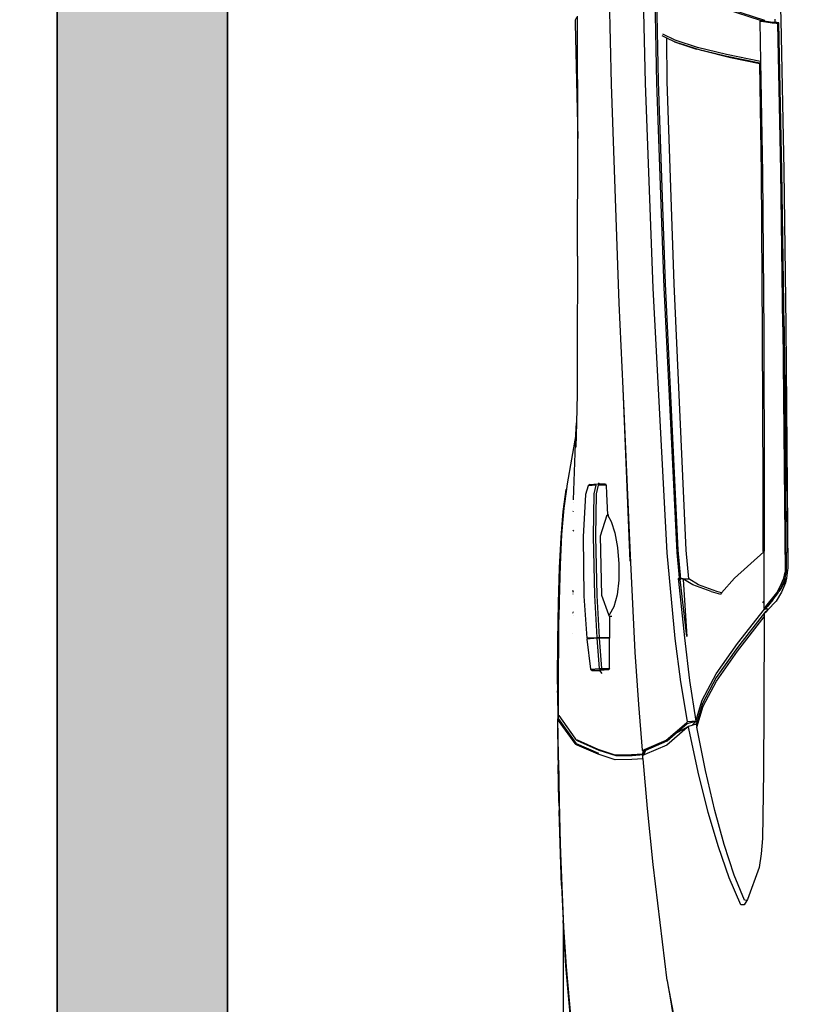
# Model space of a CAD drawing. Units: inches. Extents: x -4737294 to -4736756, y 1716389 to 1717040.
# Tile 7 of 25: x -4737217 to -4737176, y 1716491 to 1716543. Entities that reach past the tile are written whole.
import ezdxf

# ---------------------------------------------------------------- set-up
doc = ezdxf.new("R2010")
doc.units = ezdxf.units.IN
doc.header["$MEASUREMENT"] = 0
for name, color, linetype, lineweight in [('A-ANNO-DIMS', 2, 'Continuous', 18), ('A-EQPM-VEHI', 250, 'Continuous', 13), ('A-WALL-PATT', 244, 'Continuous', 13), ('walls', 252, 'Continuous', 35)]:
    doc.layers.add(name, color=color, linetype=linetype, lineweight=lineweight)
doc.layers.add('Edges', color=250, linetype='Continuous')
doc.styles.get("Standard").update_dxf_attribs({"font": 'arial.ttf'})
doc.dimstyles.get("Standard").update_dxf_attribs({"dimtxt": 8, "dimasz": 0.18, "dimexe": 0.18, "dimexo": 0.0625, "dimgap": 0.09, "dimtad": 0, "dimtih": 1, "dimtoh": 1, "dimzin": 0, "dimdsep": 46, "dimlunit": 3, "dimtxsty": 'Standard', "dimcen": 0.09, "dimadec": 0, "dimazin": 0, "dimtfac": 1, "dimtofl": 0, "dimtmove": 0, "dimatfit": 3, "dimfxl": 1, "dimtolj": 1, "dimtzin": 0, "dimarcsym": 0})

# ---------------------------------------------------------------- blocks, each defined once
blk = doc.blocks.new('Nissan Qashqai pl')
at = {"layer": 'Edges'}
for p, q in [((10.2357, 11.3043), (10.53, 11.3068)), ((10.4182, 11.3058), (10.53, 11.3068)), ((10.53, 11.3068), (10.5301, 11.3068)), ((10.5301, 11.3068), (10.5323, 11.3065)), ((10.5323, 11.3065), (10.5419, 11.3051)), ((9.696, 11.2932), (9.8644, 11.2982)), ((9.8644, 11.2982), (10.0472, 11.3018)), ((9.8681, 11.2959), (9.8678, 11.2935)), ((10.0476, 11.2996), (9.8681, 11.2959)), ((9.8681, 11.2959), (9.869, 11.2946)), ((9.869, 11.2946), (9.8689, 11.2927)), ((10.0477, 11.2982), (9.869, 11.2946)), ((10.0472, 11.3018), (10.2357, 11.3043)), ((10.2367, 11.3022), (10.0476, 11.2996)), ((10.2369, 11.3008), (10.0477, 11.2982)), ((10.2367, 11.3022), (10.5351, 11.305)), ((10.2369, 11.3008), (10.5348, 11.3036)), ((10.4153, 11.3058), (10.2954, 11.3046)), ((10.4153, 11.3058), (10.4174, 11.3058)), ((10.4174, 11.3058), (10.4181, 11.3058)), ((10.4181, 11.3058), (10.4182, 11.3058)), ((10.5422, 11.3021), (10.5348, 11.3036)), ((10.5424, 11.3035), (10.5351, 11.305)), ((10.5366, 11.3048), (10.536, 11.305)), ((10.5379, 11.3052), (10.5381, 11.305)), ((10.5419, 11.3051), (10.5463, 11.3031)), ((10.5419, 11.3051), (10.5479, 11.3042)), ((10.5522, 11.2977), (10.5422, 11.3021)), ((10.5472, 11.3014), (10.5424, 11.3035)), ((10.5463, 11.3031), (10.5551, 11.2984)), ((10.5546, 11.2982), (10.5472, 11.3014)), ((10.5479, 11.3042), (10.5589, 11.2991)), ((10.5598, 11.2935), (10.5522, 11.2977)), ((10.5583, 11.296), (10.5546, 11.2982)), ((10.5551, 11.2984), (10.5583, 11.296)), ((10.5612, 11.2944), (10.5583, 11.296)), ((10.5589, 11.2991), (10.57, 11.2925)), ((10.5683, 11.2885), (10.5612, 11.2944)), ((9.8637, 11.291), (9.8643, 11.291)), ((9.8643, 11.291), (9.8677, 11.291)), ((9.8675, 11.2887), (9.8655, 11.2754)), ((9.8686, 11.2879), (9.8665, 11.2747)), ((9.8677, 11.291), (9.8675, 11.2887)), ((9.8678, 11.2935), (9.8677, 11.291)), ((9.8689, 11.2927), (9.8686, 11.2879)), ((10.5764, 11.28), (10.5598, 11.2935)), ((10.5683, 11.2885), (10.573, 11.285)), ((10.575, 11.2829), (10.5683, 11.2885)), ((10.57, 11.2925), (10.5811, 11.2822)), ((10.573, 11.285), (10.5769, 11.2818)), ((10.5776, 11.2808), (10.575, 11.2829)), ((10.5796, 11.2824), (10.5796, 11.2787)), ((10.5811, 11.2822), (10.5821, 11.2808)), ((10.5811, 11.2822), (10.5834, 11.28)), ((9.8652, 11.2788), (9.8516, 11.2363)), ((9.8652, 11.2738), (9.8516, 11.2313)), ((9.8652, 11.2738), (9.8652, 11.2788)), ((9.8655, 11.2754), (9.8652, 11.2738)), ((9.8652, 11.2735), (9.8665, 11.2747)), ((9.8652, 11.2738), (9.8652, 11.2738)), ((9.8652, 11.2738), (9.8652, 11.2735)), ((9.8652, 11.2735), (9.8664, 11.2728)), ((9.8665, 11.2747), (9.8664, 11.2728)), ((9.8664, 11.2728), (9.9149, 11.2736)), ((9.9149, 11.2736), (9.9066, 11.2322)), ((9.9169, 11.2728), (9.9086, 11.2313)), ((9.9177, 11.2728), (9.9106, 11.2373)), ((9.9149, 11.2736), (10.0505, 11.276)), ((9.9177, 11.2728), (9.9169, 11.2728)), ((10.0501, 11.2747), (9.9177, 11.2728)), ((10.2453, 11.2762), (10.0501, 11.2747)), ((10.0505, 11.276), (10.2453, 11.2777)), ((10.2453, 11.2777), (10.4289, 11.2783)), ((10.4292, 11.2767), (10.2453, 11.2762)), ((10.4289, 11.2783), (10.5092, 11.2783)), ((10.5099, 11.2768), (10.4292, 11.2767)), ((10.5099, 11.2768), (10.5092, 11.2783)), ((10.5092, 11.2783), (10.5094, 11.2783)), ((10.5094, 11.2783), (10.51, 11.2776)), ((10.5783, 11.2783), (10.5094, 11.2783)), ((10.51, 11.2776), (10.5099, 11.2768)), ((10.51, 11.2776), (10.5419, 11.2423)), ((10.5705, 11.2771), (10.5709, 11.2767)), ((10.5709, 11.2767), (10.5719, 11.2759)), ((10.5783, 11.2783), (10.5764, 11.28)), ((10.5796, 11.2787), (10.5776, 11.2808)), ((10.5776, 11.2808), (10.5783, 11.2783)), ((10.5796, 11.2787), (10.5783, 11.2783)), ((10.6215, 11.2456), (10.5796, 11.2787)), ((10.5821, 11.2808), (10.5834, 11.2793)), ((10.5825, 11.2806), (10.5834, 11.2793)), ((10.5834, 11.28), (10.5851, 11.2783)), ((10.5834, 11.2793), (10.5835, 11.2793)), ((10.5835, 11.2793), (10.584, 11.2787)), ((10.584, 11.2789), (10.584, 11.2793)), ((10.584, 11.2787), (10.584, 11.2789)), ((10.584, 11.2787), (10.6261, 11.2458)), ((10.584, 11.2787), (10.5851, 11.2783)), ((10.5843, 11.2787), (10.584, 11.2787)), ((10.5847, 11.2787), (10.5843, 11.2787)), ((10.5851, 11.2783), (10.5892, 11.2783)), ((10.6306, 11.2459), (10.5892, 11.2783)), ((10.5892, 11.2783), (10.6988, 11.2779)), ((10.6988, 11.2779), (10.7769, 11.2774)), ((10.7769, 11.2774), (10.858, 11.2759)), ((10.858, 11.2759), (10.8766, 11.2745)), ((10.8766, 11.2745), (10.8932, 11.2722)), ((10.8932, 11.2722), (10.932, 11.258)), ((10.932, 11.258), (10.9335, 11.257)), ((10.933, 11.2541), (10.9026, 11.2417)), ((10.9384, 11.2497), (10.9059, 11.2355)), ((10.9335, 11.257), (10.933, 11.2541)), ((10.9335, 11.257), (10.9386, 11.2537)), ((10.9386, 11.2537), (10.9384, 11.2497)), ((9.9106, 11.2373), (9.9018, 11.2021)), ((10.5419, 11.2423), (10.56, 11.2265)), ((10.6583, 11.2197), (10.6215, 11.2456)), ((10.6261, 11.2458), (10.6627, 11.22)), ((10.6671, 11.2203), (10.6306, 11.2459)), ((10.9026, 11.2417), (10.8653, 11.2297)), ((10.9059, 11.2355), (10.8682, 11.2226)), ((9.9066, 11.2322), (9.8978, 11.197)), ((9.9086, 11.2313), (9.8998, 11.196)), ((10.56, 11.2265), (10.5584, 11.2206)), ((10.5584, 11.2136), (10.5617, 11.2251)), ((10.56, 11.2265), (10.5617, 11.2251)), ((10.8653, 11.2297), (10.8239, 11.2181)), ((10.8682, 11.2226), (10.8264, 11.21)), ((10.5584, 11.2206), (10.5502, 11.1986)), ((10.5584, 11.2136), (10.5502, 11.1916)), ((10.69, 11.2028), (10.6583, 11.2197)), ((10.6627, 11.22), (10.6943, 11.2032)), ((10.6976, 11.2041), (10.6671, 11.2203)), ((10.8239, 11.2181), (10.7754, 11.2071)), ((9.9018, 11.2021), (9.8931, 11.1752)), ((10.5502, 11.1986), (10.543, 11.1865)), ((10.7155, 11.1952), (10.69, 11.2028)), ((10.6943, 11.2032), (10.7155, 11.1969)), ((10.7228, 11.1965), (10.6976, 11.2041)), ((10.7754, 11.2071), (10.7228, 11.1965)), ((10.8264, 11.21), (10.7776, 11.1982)), ((9.8978, 11.197), (9.8891, 11.1701)), ((9.8911, 11.1693), (9.8998, 11.196)), ((10.543, 11.1865), (10.5079, 11.1835)), ((10.5502, 11.1916), (10.543, 11.1795)), ((10.543, 11.1795), (10.543, 11.1865)), ((10.6144, 11.1813), (10.6664, 11.1875)), ((10.6664, 11.1875), (10.7155, 11.1952)), ((10.7155, 11.1957), (10.7155, 11.1969)), ((10.7155, 11.1969), (10.7192, 11.1957)), ((10.7209, 11.1902), (10.7155, 11.1957)), ((10.7155, 11.1952), (10.7155, 11.1957)), ((10.7186, 11.1848), (10.7155, 11.1952)), ((10.7155, 11.1952), (10.7165, 11.1851)), ((10.7192, 11.1957), (10.7228, 11.1965)), ((10.7192, 11.1957), (10.7209, 11.1902)), ((10.7209, 11.1902), (10.7221, 11.1861)), ((10.7247, 11.1867), (10.7222, 11.186)), ((10.7776, 11.1982), (10.7247, 11.1867)), ((9.8931, 11.1751), (9.8911, 11.1693)), ((9.8931, 11.1751), (9.8931, 11.1752)), ((10.5079, 11.1835), (10.1849, 11.1687)), ((10.543, 11.1771), (10.5079, 11.1739)), ((10.5109, 11.1721), (10.5417, 11.1748)), ((10.543, 11.1771), (10.5417, 11.1748)), ((10.5417, 11.1748), (10.5427, 11.1739)), ((10.5436, 11.1754), (10.5427, 11.1739)), ((10.5439, 11.1796), (10.543, 11.1795)), ((10.543, 11.1795), (10.543, 11.1771)), ((10.544, 11.1763), (10.543, 11.1771)), ((10.544, 11.1763), (10.5436, 11.1754)), ((10.5439, 11.1796), (10.613, 11.1841)), ((10.547, 11.1767), (10.544, 11.1763)), ((10.5458, 11.1742), (10.6144, 11.1813)), ((10.613, 11.1841), (10.547, 11.1767)), ((10.6678, 11.177), (10.6152, 11.1702)), ((10.7137, 11.1846), (10.6678, 11.177)), ((10.7165, 11.1851), (10.7137, 11.1846)), ((10.7177, 11.1838), (10.7165, 11.1851)), ((10.7387, 11.1593), (10.7177, 11.1838)), ((10.7312, 11.1701), (10.7186, 11.1848)), ((10.7221, 11.1861), (10.7222, 11.1859)), ((10.7222, 11.186), (10.7221, 11.1861)), ((10.7222, 11.186), (10.7222, 11.1859)), ((10.7222, 11.1859), (10.7232, 11.1848)), ((10.7222, 11.1859), (10.7224, 11.1855)), ((10.7224, 11.1855), (10.7312, 11.1701)), ((10.7232, 11.1848), (10.7228, 11.1859)), ((10.7232, 11.1848), (10.7449, 11.1598)), ((10.7257, 11.1853), (10.7256, 11.1854)), ((11.0357, 11.1613), (11.1598, 11.1847)), ((11.0492, 11.1635), (11.1336, 11.1772)), ((9.8891, 11.1701), (9.8818, 11.1551)), ((9.8911, 11.1691), (9.8867, 11.16)), ((9.8911, 11.1693), (9.8911, 11.1691)), ((10.1849, 11.1687), (9.9393, 11.1602)), ((10.5079, 11.1739), (10.1849, 11.1585)), ((10.1894, 11.1563), (10.5109, 11.1721)), ((10.6152, 11.1702), (10.5113, 11.1603)), ((10.5427, 11.1739), (10.5458, 11.1742)), ((10.7397, 11.1602), (10.7312, 11.1701)), ((11.0357, 11.1613), (11.0491, 11.1635)), ((11.0492, 11.1635), (11.0491, 11.1635)), ((9.8867, 11.16), (9.8838, 11.1541)), ((9.9393, 11.1602), (9.8867, 11.16)), ((10.1849, 11.1585), (9.9393, 11.1497)), ((9.9411, 11.1475), (10.1894, 11.1563)), ((10.5113, 11.1603), (10.19, 11.1433)), ((10.7501, 11.1327), (10.7387, 11.1593)), ((10.7507, 11.1344), (10.7397, 11.1602)), ((10.7449, 11.1598), (10.7563, 11.1333)), ((11.0304, 11.1603), (10.8896, 11.1434)), ((11.0304, 11.1603), (11.0357, 11.1613)), ((9.8101, 11.1449), (9.9411, 11.1475)), ((9.9393, 11.1497), (9.8119, 11.1472)), ((10.19, 11.1433), (9.9414, 11.1341)), ((10.8896, 11.1434), (10.8218, 11.1365)), ((9.9414, 11.1341), (9.8143, 11.1312)), ((10.6955, 11.1257), (10.7509, 11.1302)), ((10.7507, 11.1309), (10.7501, 11.1327)), ((10.7511, 11.1335), (10.7507, 11.1344)), ((10.7507, 11.1344), (10.7524, 11.1335)), ((10.751, 11.131), (10.7507, 11.1309)), ((10.7509, 11.1302), (10.7507, 11.1309)), ((10.7522, 11.1311), (10.7509, 11.1302)), ((10.7516, 11.131), (10.7509, 11.1302)), ((10.7519, 11.1314), (10.7511, 11.1335)), ((10.7519, 11.1314), (10.7516, 11.131)), ((10.7522, 11.1311), (10.7516, 11.131)), ((10.7526, 11.1318), (10.7519, 11.1314)), ((10.7553, 11.1307), (10.7522, 11.1311)), ((10.7524, 11.1335), (10.7526, 11.1318)), ((10.7524, 11.1335), (10.7556, 11.1319)), ((10.7532, 11.1321), (10.7526, 11.1318)), ((10.7526, 11.1318), (10.7526, 11.1314)), ((10.7556, 11.1319), (10.7532, 11.1321)), ((10.7563, 11.1169), (10.7553, 11.1307)), ((10.7556, 11.1319), (10.7561, 11.1317)), ((10.7563, 11.1319), (10.7561, 11.1319)), ((10.7563, 11.1315), (10.7561, 11.1317)), ((10.7561, 11.1317), (10.7563, 11.1317)), ((10.7563, 11.1333), (10.7569, 11.1317)), ((10.7563, 11.1317), (10.7563, 11.1319)), ((10.7563, 11.1317), (10.7569, 11.1317)), ((10.7569, 11.1316), (10.7563, 11.1317)), ((10.7563, 11.1315), (10.7563, 11.1317)), ((10.7572, 11.1178), (10.7563, 11.1315)), ((10.7573, 11.1307), (10.7563, 11.1315)), ((10.7569, 11.1317), (10.7569, 11.1316)), ((10.7569, 11.1316), (10.7573, 11.1307)), ((10.7604, 11.131), (10.7573, 11.1307)), ((10.7615, 11.1311), (10.7604, 11.131)), ((10.8218, 11.1365), (10.7615, 11.1311)), ((10.7615, 11.1311), (10.7623, 11.1173)), ((10.312, 11.1064), (10.5147, 11.1156)), ((10.312, 11.1064), (10.5214, 11.1149)), ((10.5147, 11.1156), (10.6318, 11.1213)), ((10.6318, 11.1213), (10.6955, 11.1257)), ((10.7565, 11.0969), (10.7563, 11.1169)), ((10.7575, 11.0979), (10.7572, 11.1178)), ((10.7623, 11.1173), (10.7626, 11.0974)), ((10.2081, 11.1017), (10.312, 11.1064)), ((9.8024, 11.0892), (9.9426, 11.0923)), ((9.9426, 11.0923), (10.2081, 11.1017)), ((10.4653, 11.0881), (10.4732, 11.0925)), ((10.4732, 11.0925), (10.4871, 11.0967)), ((10.4871, 11.0967), (10.5048, 11.1002)), ((10.5048, 11.1002), (10.5246, 11.1019)), ((10.5246, 11.1019), (10.5445, 11.1017)), ((10.5445, 11.1017), (10.5625, 11.0996)), ((10.5625, 11.0996), (10.5769, 11.0957)), ((10.5769, 11.0957), (10.5863, 11.0904)), ((10.5885, 11.0931), (10.5885, 11.0904)), ((10.7497, 11.0763), (10.7565, 11.0969)), ((10.7507, 11.0773), (10.7575, 11.0979)), ((10.7626, 11.0974), (10.7559, 11.0767)), ((10.4274, 11.0767), (10.4275, 11.0856)), ((10.4275, 11.0856), (10.4293, 11.0863)), ((10.4293, 11.0863), (10.4291, 11.0765)), ((10.4293, 11.0863), (10.4398, 11.0868)), ((10.4398, 11.0868), (10.4653, 11.0878)), ((10.4653, 11.0881), (10.4652, 11.0897)), ((10.4653, 11.0877), (10.4653, 11.0881)), ((10.4653, 11.0878), (10.4653, 11.0881)), ((10.4653, 11.0881), (10.4653, 11.0881)), ((10.4653, 11.0877), (10.4653, 11.0878)), ((10.4908, 11.0793), (10.4653, 11.0877)), ((10.563, 11.0809), (10.4908, 11.0793)), ((10.5867, 11.0897), (10.563, 11.0809)), ((10.5863, 11.0904), (10.5867, 11.0897)), ((10.5885, 11.0904), (10.5867, 11.0897)), ((10.5885, 11.0904), (10.6141, 11.0905)), ((10.6141, 11.0905), (10.615, 11.0905)), ((10.6142, 11.0782), (10.6141, 11.0905)), ((10.6517, 11.0902), (10.615, 11.0905)), ((10.615, 11.0905), (10.6151, 11.0782)), ((10.6151, 11.078), (10.6518, 11.0808)), ((10.6518, 11.0808), (10.6517, 11.0902)), ((10.6517, 11.0902), (10.6535, 11.0895)), ((10.6518, 11.0784), (10.6518, 11.0808)), ((10.6518, 11.0808), (10.6536, 11.0803)), ((10.6536, 11.0803), (10.6518, 11.0784)), ((10.6535, 11.0895), (10.6543, 11.0786)), ((10.6535, 11.0895), (10.6536, 11.0803)), ((10.6536, 11.0803), (10.6537, 11.0783)), ((10.6578, 11.0814), (10.6543, 11.0786)), ((10.4263, 11.0777), (10.4274, 11.0767)), ((10.4274, 11.0762), (10.4274, 11.0767)), ((10.4282, 11.0666), (10.4274, 11.0762)), ((10.4291, 11.0765), (10.4398, 11.0741)), ((10.4398, 11.0718), (10.4291, 11.0741)), ((10.4291, 11.0741), (10.4299, 11.0644)), ((10.4398, 11.0741), (10.4909, 11.0734)), ((10.4909, 11.0711), (10.4398, 11.0718)), ((10.4909, 11.0734), (10.563, 11.075)), ((10.5631, 11.0727), (10.4909, 11.0711)), ((10.563, 11.075), (10.6142, 11.0779)), ((10.6142, 11.0756), (10.5631, 11.0727)), ((10.6142, 11.0779), (10.6142, 11.0782)), ((10.6142, 11.0765), (10.6142, 11.0779)), ((10.615, 11.0765), (10.6142, 11.0765)), ((10.6142, 11.0756), (10.6142, 11.0765)), ((10.615, 11.0639), (10.6142, 11.0756)), ((10.6151, 11.0765), (10.615, 11.0765)), ((10.615, 11.0765), (10.6151, 11.0639)), ((10.6518, 11.0784), (10.6151, 11.0756)), ((10.6151, 11.0782), (10.6151, 11.078)), ((10.6151, 11.078), (10.6151, 11.0765)), ((10.6151, 11.0765), (10.6151, 11.0756)), ((10.6151, 11.0756), (10.616, 11.0629)), ((10.616, 11.0629), (10.6526, 11.0674)), ((10.6526, 11.0674), (10.6518, 11.0784)), ((10.6526, 11.0674), (10.6543, 11.0693)), ((10.6543, 11.0786), (10.6537, 11.0783)), ((10.6537, 11.0783), (10.6543, 11.0693)), ((10.6543, 11.0693), (10.6543, 11.0786)), ((10.7385, 11.051), (10.7497, 11.0763)), ((10.7396, 11.0519), (10.7507, 11.0773)), ((10.7549, 11.0776), (10.743, 11.0503)), ((10.7559, 11.0767), (10.7448, 11.0511)), ((10.4282, 11.0666), (10.4299, 11.0644)), ((10.4299, 11.0644), (10.4406, 11.0612)), ((10.4406, 11.0612), (10.4919, 11.0584)), ((10.4919, 11.0584), (10.564, 11.0591)), ((10.564, 11.0591), (10.6151, 11.0628)), ((10.6151, 11.0639), (10.615, 11.0639)), ((10.6151, 11.0628), (10.615, 11.0639)), ((10.6151, 11.0639), (10.6151, 11.0628)), ((9.8643, 11.0514), (9.8598, 11.0514)), ((9.8614, 11.0504), (9.8647, 11.0485)), ((10.0085, 11.0519), (9.8643, 11.0514)), ((9.8647, 11.0485), (9.869, 11.0488)), ((9.869, 11.0488), (10.0085, 11.0519)), ((10.0124, 11.0519), (10.0085, 11.0519)), ((10.1513, 11.0517), (10.0124, 11.0519)), ((10.1513, 11.0517), (10.2677, 11.0512)), ((10.2677, 11.0512), (10.3189, 11.0511)), ((10.3189, 11.0511), (10.3537, 11.0503)), ((10.3537, 11.0503), (10.3832, 11.0496)), ((10.3679, 11.0497), (10.3537, 11.0503)), ((10.3679, 11.0497), (10.4275, 11.0391)), ((10.4468, 11.0466), (10.3679, 11.0497)), ((10.4502, 11.0466), (10.4503, 11.0465)), ((10.4613, 11.0464), (10.4603, 11.0465)), ((10.4838, 11.0465), (10.4852, 11.046)), ((10.5565, 11.0456), (10.5591, 11.0464)), ((10.5615, 11.0464), (10.5617, 11.0457)), ((10.583, 11.0457), (10.5835, 11.0461)), ((10.5836, 11.0461), (10.5832, 11.0457)), ((10.5847, 11.0461), (10.5841, 11.0457)), ((10.5873, 11.0461), (10.5873, 11.0461)), ((10.6087, 11.0458), (10.6087, 11.0458)), ((10.7087, 11.0289), (10.7363, 11.0483)), ((10.7424, 11.0499), (10.7125, 11.0285)), ((10.7429, 11.0485), (10.7148, 11.0284)), ((10.7363, 11.0483), (10.7376, 11.0492)), ((10.7387, 11.0502), (10.7376, 11.0492)), ((10.7376, 11.0492), (10.7378, 11.0495)), ((10.7378, 11.0495), (10.7385, 11.051)), ((10.7378, 11.0495), (10.7379, 11.0496)), ((10.7387, 11.0502), (10.7396, 11.0519)), ((10.7424, 11.0499), (10.743, 11.0503)), ((10.7429, 11.0488), (10.7432, 11.0488)), ((10.7432, 11.0488), (10.7429, 11.0485)), ((10.744, 11.0494), (10.7432, 11.0488)), ((10.7448, 11.0511), (10.744, 11.0494)), ((11.0798, 11.0434), (11.0576, 11.0416)), ((11.059, 11.0419), (11.0768, 11.0434)), ((10.4275, 11.0391), (10.4304, 11.0385)), ((10.4304, 11.0385), (10.4339, 11.0381)), ((10.4345, 11.0379), (10.4339, 11.0381)), ((10.4339, 11.0381), (10.4573, 11.0349)), ((10.4613, 11.0343), (10.4345, 11.0379)), ((10.4573, 11.0349), (10.4889, 11.0323)), ((10.4926, 11.0317), (10.4613, 11.0343)), ((10.4889, 11.0323), (10.526, 11.0304)), ((10.5294, 11.0298), (10.4926, 11.0317)), ((10.9152, 11.0321), (10.8642, 11.0304)), ((10.8642, 11.0305), (10.8759, 11.031)), ((10.8644, 11.0306), (10.8759, 11.031)), ((10.8759, 11.031), (10.9158, 11.0324)), ((10.9152, 11.0321), (10.9577, 11.0341)), ((10.9158, 11.0324), (10.9657, 11.0347)), ((10.9649, 11.0344), (10.9577, 11.0341)), ((10.9577, 11.0341), (11.1283, 11.0341)), ((11.0127, 11.0375), (10.9649, 11.0344)), ((10.9657, 11.0347), (11.0138, 11.0377)), ((11.0576, 11.0416), (11.0127, 11.0375)), ((11.0138, 11.0377), (11.059, 11.0419)), ((10.526, 11.0304), (10.569, 11.0291)), ((10.5719, 11.0285), (10.5294, 11.0298)), ((10.569, 11.0291), (10.5919, 11.0287)), ((10.6176, 11.0277), (10.5719, 11.0285)), ((10.5919, 11.0287), (10.5936, 11.0286)), ((10.5936, 11.0286), (10.6151, 11.0283)), ((10.6151, 11.0283), (10.6644, 11.028)), ((10.6651, 11.0274), (10.6176, 11.0277)), ((10.6644, 11.028), (10.7078, 11.0282)), ((10.677, 11.0275), (10.6651, 11.0274)), ((10.7082, 11.0285), (10.6729, 11.0284)), ((10.68, 11.0274), (10.677, 11.0275)), ((10.6809, 11.0274), (10.68, 11.0274)), ((10.6809, 11.0274), (10.7128, 11.0275)), ((10.7078, 11.0282), (10.7083, 11.0285)), ((10.7082, 11.0285), (10.7078, 11.0282)), ((10.7085, 11.0289), (10.7082, 11.0285)), ((10.7083, 11.0285), (10.7082, 11.0285)), ((10.7083, 11.0285), (10.7087, 11.0289)), ((10.7125, 11.0285), (10.7083, 11.0285)), ((10.7146, 11.0286), (10.7125, 11.0285)), ((10.7125, 11.0285), (10.7139, 11.0278)), ((10.7134, 11.0275), (10.7128, 11.0275)), ((10.7625, 11.0281), (10.7134, 11.0275)), ((10.724, 11.0275), (10.7134, 11.0275)), ((10.7148, 11.0284), (10.7139, 11.0278)), ((10.7628, 11.0283), (10.7139, 11.0278)), ((10.724, 11.0275), (10.7685, 11.0281)), ((10.7628, 11.0281), (10.7625, 11.0281)), ((10.7628, 11.0283), (10.8131, 11.0292)), ((10.7628, 11.0281), (10.8131, 11.029)), ((10.7688, 11.0281), (10.7685, 11.0281)), ((10.8131, 11.029), (10.7688, 11.0281)), ((10.8131, 11.0292), (10.8644, 11.0306)), ((10.8132, 11.029), (10.8131, 11.029)), ((10.8132, 11.029), (10.8139, 11.029)), ((10.8142, 11.029), (10.8139, 11.029)), ((10.8142, 11.029), (10.8241, 11.0293)), ((10.8142, 11.029), (10.8142, 11.029)), ((10.8242, 11.0293), (10.8241, 11.0293)), ((10.8246, 11.0293), (10.8242, 11.0293)), ((10.8642, 11.0304), (10.8246, 11.0293))]:
    blk.add_line(p, q, dxfattribs=at)
blk = doc.blocks.new('car')
blk.add_blockref('Nissan Qashqai pl', (-9.7433, -11.9151))
blk = doc.blocks.new('*D59')
at = {"layer": 'A-ANNO-DIMS', "color": 0, "lineweight": -2, "transparency": 16777216}
for p, q in [((-4737196.539, 1716655.661), (-4737225.279, 1716655.661)), ((-4737225.099, 1716655.481), (-4737225.099, 1716564.479)), ((-4737225.099, 1716465.024), (-4737225.099, 1716556.026)), ((-4737196.539, 1716464.844), (-4737225.279, 1716464.844))]:
    blk.add_line(p, q, dxfattribs=at)
at = {"layer": 'A-ANNO-DIMS', "color": 0, "transparency": 16777216}
for points in [[(-4737225.129, 1716655.481), (-4737225.069, 1716655.481), (-4737225.099, 1716655.661)], [(-4737225.129, 1716465.024), (-4737225.069, 1716465.024), (-4737225.099, 1716464.844)]]:
    blk.add_solid(points, dxfattribs=at)
at = {"layer": 'Defpoints', "color": 0, "transparency": 16777216}
for p in [(-4737196.476, 1716655.661), (-4737225.099, 1716464.844), (-4737196.476, 1716464.844)]:
    blk.add_point(p, dxfattribs=at)
at = {"layer": 'A-ANNO-DIMS', "color": 0, "transparency": 16777216, "insert": (-4737225.099, 1716560.253), "char_height": 8, "attachment_point": 5}
blk.add_mtext('\\A1;CAR 15\'-11"', dxfattribs=at)

msp = doc.modelspace()

# ---------------------------------------------------------------- hatches: boundary and pattern name
at = {"layer": 'A-WALL-PATT'}
h = msp.add_hatch(color=256, dxfattribs=at)
h.dxf.hatch_style = 1
h.paths.add_polyline_path([(-4737206.144, 1716844.565), (-4737110.144, 1716844.565), (-4737110.144, 1716823.907), (-4737105.644, 1716823.907), (-4737105.644, 1716844.565), (-4737098.44, 1716844.565), (-4737098.44, 1716849.065), (-4737206.144, 1716849.065), (-4737206.144, 1716993.065), (-4736864.144, 1716993.065), (-4736864.144, 1716849.065), (-4736963.275, 1716849.065), (-4736994.446, 1716849.065), (-4736997.144, 1716849.065), (-4736997.144, 1716844.565), (-4736864.144, 1716844.565), (-4736864.144, 1716668.565), (-4736934.391, 1716668.565), (-4736934.391, 1716664.065), (-4736864.144, 1716664.065), (-4736864.144, 1716462.065), (-4736855.144, 1716462.065), (-4736855.144, 1717002.065), (-4737215.144, 1717002.065), (-4737215.144, 1716462.065), (-4737206.144, 1716462.065), (-4737206.144, 1716659.065), (-4737062.144, 1716659.065), (-4737062.144, 1716647.493), (-4737057.644, 1716647.493), (-4737057.644, 1716796.565), (-4737071.812, 1716796.565), (-4737071.812, 1716792.065), (-4737070.805, 1716792.065), (-4737062.144, 1716792.065), (-4737062.144, 1716668.065), (-4737206.144, 1716668.065), (-4737206.144, 1716792.065), (-4737093.784, 1716792.065), (-4737093.784, 1716796.565), (-4737206.144, 1716796.565)])

# ---------------------------------------------------------------- linework, layer by layer
at = {"layer": 'walls'}
for p, q in [((-4737215.144, 1716462.065), (-4737215.144, 1717002.065)), ((-4737206.144, 1716462.065), (-4737206.144, 1716659.065))]:
    msp.add_line(p, q, dxfattribs=at)

# ---------------------------------------------------------------- block references
at = {"layer": 'A-EQPM-VEHI', "xscale": 43.56002006885659, "yscale": 43.56002006885659, "zscale": 43.56002006885659, "rotation": 270}
msp.add_blockref('car', (-4737150.017, 1716548.61), dxfattribs=at)

# ---------------------------------------------------------------- dimensions: what is measured, and where the dimension line sits
at = {"layer": 'A-ANNO-DIMS'}
dim = msp.add_linear_dim(base=(-4737225.099, 1716464.844), p1=(-4737196.476, 1716655.661), p2=(-4737196.476, 1716464.844), angle=270, text='CAR <>', dimstyle='Standard', override={"dimdec": 1, "dimlfac": 1, "dimrnd": 0, "dimzin": 1, "dimdsep": 46, "dimlunit": 4, "dimfrac": 2}, dxfattribs=at)
dim.commit()
dim.dimension.update_dxf_attribs({"geometry": '*D59', "text_midpoint": (-4737225.099, 1716560.253)})

doc.saveas('drawing.dxf')
